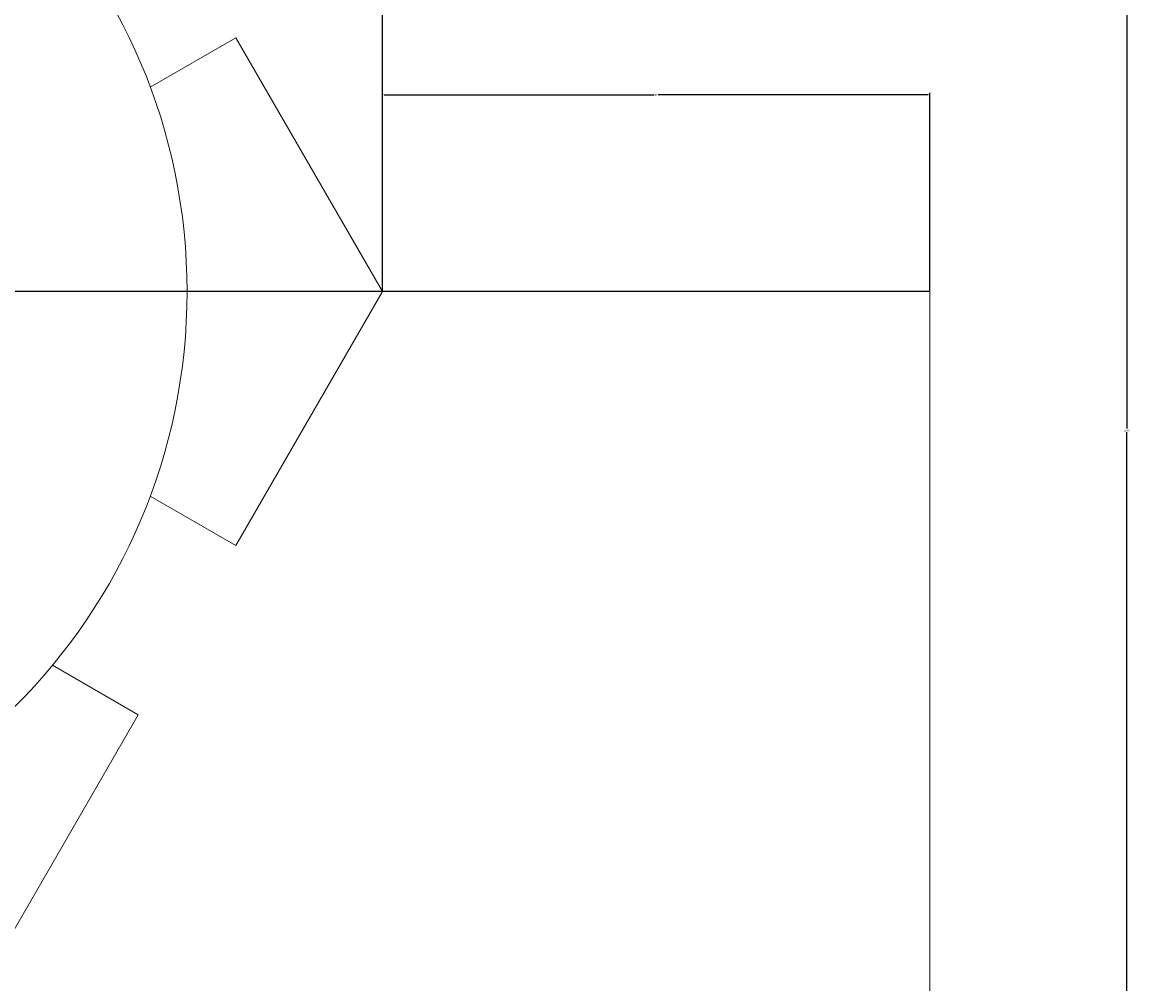
# Model space of a CAD drawing. Units: inches. Extents: x 1095 to 1408, y -20 to 240.
# Tile 7 of 8: x 1294 to 1408, y 53 to 152. Entities that reach past the tile are written whole.
import ezdxf

# ---------------------------------------------------------------- set-up
doc = ezdxf.new("R2010")
doc.units = ezdxf.units.IN
doc.header["$MEASUREMENT"] = 0
doc.layers.add('M-CONS', color=8, linetype='Continuous', lineweight=18)
doc.layers.add('M-DIMS', color=2, linetype='Continuous', lineweight=18)
doc.styles.get("Standard").update_dxf_attribs({"font": 'arial.ttf'})
doc.dimstyles.get("Standard").update_dxf_attribs({"dimtxt": 0.18, "dimasz": 0.18, "dimexe": 0.18, "dimexo": 0.0625, "dimgap": 0.09, "dimtad": 0, "dimtih": 1, "dimtoh": 1, "dimdec": 4, "dimzin": 0, "dimdsep": 46, "dimtxsty": 'Standard', "dimcen": 0.09, "dimadec": 0, "dimazin": 0, "dimtfac": 1, "dimtdec": 4, "dimtofl": 0, "dimtmove": 0, "dimatfit": 3, "dimfxl": 1, "dimtolj": 1, "dimtzin": 0, "dimarcsym": 0})

# ---------------------------------------------------------------- blocks, each defined once
blk = doc.blocks.new('*D2')
at = {"layer": 'Defpoints', "color": 0, "transparency": 16777216}
for p in [(1365.18, 219.6), (1407.33, 219.6), (1387.18, 0)]:
    blk.add_point(p, dxfattribs=at)
at = {"layer": 'M-DIMS', "color": 0, "lineweight": -2, "transparency": 16777216}
for p, q in [((1365.25, 219.6), (1407.51, 219.6)), ((1407.33, 219.42), (1407.33, 109.98)), ((1407.33, 0.18), (1407.33, 109.62)), ((1387.25, 0), (1407.51, 0))]:
    blk.add_line(p, q, dxfattribs=at)
at = {"layer": 'M-DIMS', "color": 0, "transparency": 16777216}
for points in [[(1407.3, 219.42), (1407.36, 219.42), (1407.33, 219.6)], [(1407.3, 0.18), (1407.36, 0.18), (1407.33, 0)]]:
    blk.add_solid(points, dxfattribs=at)
at = {"layer": 'M-DIMS', "color": 0, "transparency": 16777216, "insert": (1407.33, 109.8), "char_height": 0.18, "attachment_point": 5}
blk.add_mtext('\\A1;219.6', dxfattribs=at)
blk = doc.blocks.new('*D7')
at = {"layer": 'Defpoints', "color": 0, "transparency": 16777216}
for p in [(1387.18, 144.15), (1331.18, 124), (1387.18, 124)]:
    blk.add_point(p, dxfattribs=at)
at = {"layer": 'M-DIMS', "color": 0, "lineweight": -2, "transparency": 16777216}
for p, q in [((1331.18, 124.06), (1331.18, 144.33)), ((1331.36, 144.15), (1358.96, 144.15)), ((1387, 144.15), (1359.4, 144.15)), ((1387.18, 124.06), (1387.18, 144.33))]:
    blk.add_line(p, q, dxfattribs=at)
at = {"layer": 'M-DIMS', "color": 0, "transparency": 16777216}
for points in [[(1331.36, 144.18), (1331.36, 144.12), (1331.18, 144.15)], [(1387, 144.18), (1387, 144.12), (1387.18, 144.15)]]:
    blk.add_solid(points, dxfattribs=at)
at = {"layer": 'M-DIMS', "color": 0, "transparency": 16777216, "insert": (1359.18, 144.15), "char_height": 0.18, "attachment_point": 5}
blk.add_mtext('\\A1;56', dxfattribs=at)
blk = doc.blocks.new('*D8')
at = {"layer": 'Defpoints', "color": 0, "transparency": 16777216}
for p in [(1095.03, 124), (1387.18, 124), (1365.18, 40)]:
    blk.add_point(p, dxfattribs=at)
at = {"layer": 'M-DIMS', "color": 0, "lineweight": -2, "transparency": 16777216}
for p, q in [((1387.12, 124), (1094.85, 124)), ((1095.03, 123.82), (1095.03, 82.18)), ((1095.03, 40.18), (1095.03, 81.82)), ((1365.12, 40), (1094.85, 40))]:
    blk.add_line(p, q, dxfattribs=at)
at = {"layer": 'M-DIMS', "color": 0, "transparency": 16777216}
for points in [[(1095, 123.82), (1095.06, 123.82), (1095.03, 124)], [(1095, 40.18), (1095.06, 40.18), (1095.03, 40)]]:
    blk.add_solid(points, dxfattribs=at)
at = {"layer": 'M-DIMS', "color": 0, "transparency": 16777216, "insert": (1095.03, 82), "char_height": 0.18, "attachment_point": 5}
blk.add_mtext('\\A1;84', dxfattribs=at)
blk = doc.blocks.new('*D9')
at = {"layer": 'Defpoints', "color": 0, "transparency": 16777216}
for p in [(1331.18, 239.75), (1171.18, 124), (1331.18, 124)]:
    blk.add_point(p, dxfattribs=at)
at = {"layer": 'M-DIMS', "color": 0, "lineweight": -2, "transparency": 16777216}
for p, q in [((1171.18, 124.06), (1171.18, 239.93)), ((1171.36, 239.75), (1250.9, 239.75)), ((1331, 239.75), (1251.46, 239.75)), ((1331.18, 124.06), (1331.18, 239.93))]:
    blk.add_line(p, q, dxfattribs=at)
at = {"layer": 'M-DIMS', "color": 0, "transparency": 16777216}
for points in [[(1171.36, 239.78), (1171.36, 239.72), (1171.18, 239.75)], [(1331, 239.78), (1331, 239.72), (1331.18, 239.75)]]:
    blk.add_solid(points, dxfattribs=at)
at = {"layer": 'M-DIMS', "color": 0, "transparency": 16777216, "insert": (1251.18, 239.75), "char_height": 0.18, "attachment_point": 5}
blk.add_mtext('\\A1;160', dxfattribs=at)

msp = doc.modelspace()

# ---------------------------------------------------------------- linework, layer by layer
at = {"layer": 'M-CONS', "extrusion": (0, -1, 0)}
msp.add_line((1387.184, 0, 397.783), (1387.184, 124, 397.783), dxfattribs=at)
at = {"layer": 'M-CONS', "elevation": 377.783}
for points in [[(1307.418, 103.08), (1316.184, 98.019), (1331.184, 124), (1316.184, 149.981), (1307.418, 144.92)], [(1204.949, 85.759), (1196.184, 80.699), (1211.184, 54.718), (1291.184, 54.718), (1306.184, 80.699), (1297.418, 85.759)]]:
    msp.add_lwpolyline(points, dxfattribs=at)
at = {"layer": 'M-CONS'}
msp.add_circle((1251.184, 124, 377.783), 60, dxfattribs=at)

# ---------------------------------------------------------------- dimensions: what is measured, and where the dimension line sits
at = {"layer": 'M-DIMS'}
dim = msp.add_linear_dim(base=(1331.184, 239.75), p1=(1171.184, 124), p2=(1331.184, 124), dimstyle='Standard', override={"dimdec": 0, "dimlfac": 1, "dimrnd": 0, "dimzin": 0, "dimdsep": 46, "dimlunit": 2}, dxfattribs=at)
dim.commit()
dim.dimension.update_dxf_attribs({"geometry": '*D9', "text_midpoint": (1251.184, 239.75)})
for base, p1, p2, angle, override, picture, middle in [((1407.334, 219.6), (1387.184, 0), (1365.184, 219.6), 90, {"dimdec": 1, "dimlfac": 1, "dimrnd": 0, "dimzin": 0, "dimdsep": 46, "dimlunit": 2}, '*D2', (1407.334, 109.8)), ((1387.184, 144.15), (1331.184, 124), (1387.184, 124), 0, {"dimdec": 0, "dimlfac": 1, "dimrnd": 0, "dimzin": 0, "dimdsep": 46, "dimlunit": 2}, '*D7', (1359.184, 144.15)), ((1095.034, 124), (1365.184, 40), (1387.184, 124), 90, {"dimdec": 0, "dimlfac": 1, "dimrnd": 0, "dimzin": 0, "dimdsep": 46, "dimlunit": 2}, '*D8', (1095.034, 82))]:
    dim = msp.add_linear_dim(base=base, p1=p1, p2=p2, angle=angle, dimstyle='Standard', override=override, dxfattribs=at)
    dim.commit()
    dim.dimension.update_dxf_attribs({"geometry": picture, "text_midpoint": middle})

doc.saveas('drawing.dxf')
